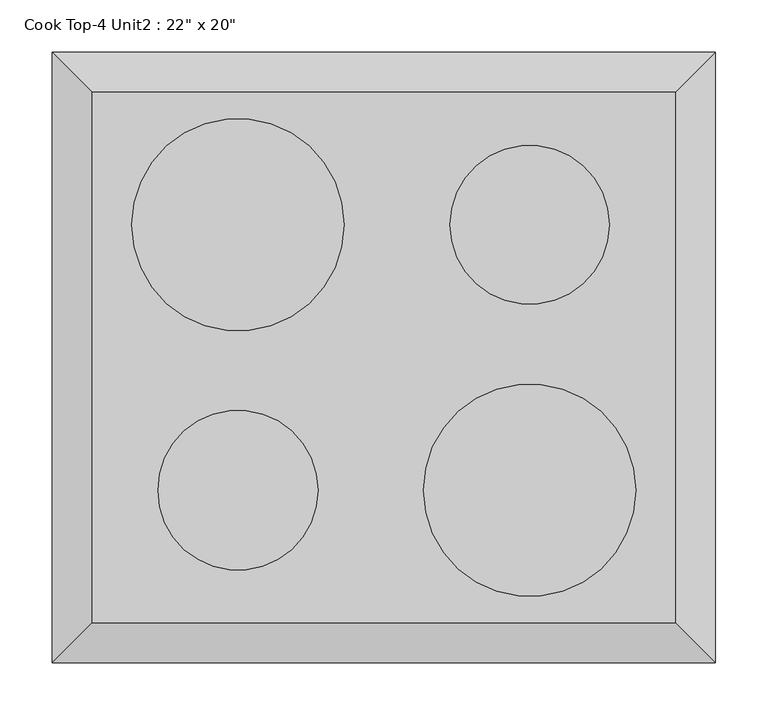
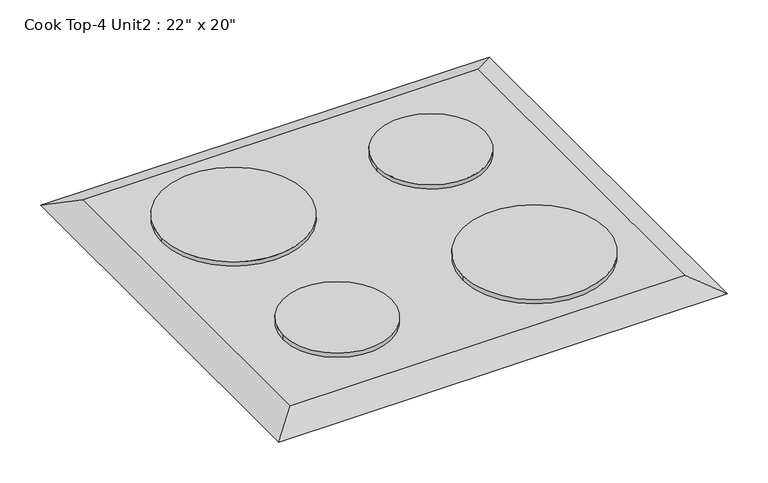
"""IFC4 building model written with IfcOpenShell, lengths in millimetres: proxy geometry."""

from ifc_helpers import new_model, si_unit, point, frame, frame_2d, origin, place, context, project, spatial, circle_curve, trimmed, segment, composite_curve, outline, extrude, faceted_brep, source, transform, mapped, element, save


def proxy_dfcd9396(model_context):
    return source(origin(), model_context, "Body", "SolidModel", [
        extrude(outline(composite_curve([segment(trimmed(circle_curve(frame_2d((-139.7, -127.0)), 76.5869489), [point((-63.1130511, -127.0))], [point((-216.2869489, -127.0))], False, "CARTESIAN"), True, "CONTINUOUS"), segment(trimmed(circle_curve(frame_2d((-139.7, -127.0)), 76.5869489), [point((-216.2869489, -127.0))], [point((-63.1130511, -127.0))], False, "CARTESIAN"), True, "CONTINUOUS")], self_intersect=False)), frame((0.0, 0.0, 918.0), z_axis=(0.0, 0.0, 1.0), x_axis=(1.0, 0.0, 0.0)), (0.0, 0.0, 1.0), 6.35),
        extrude(outline(composite_curve([segment(trimmed(circle_curve(frame_2d((139.7, 127.0)), 76.2), [point((215.9, 127.0))], [point((63.5, 127.0))], False, "CARTESIAN"), True, "CONTINUOUS"), segment(trimmed(circle_curve(frame_2d((139.7, 127.0)), 76.2), [point((63.5, 127.0))], [point((215.9, 127.0))], False, "CARTESIAN"), True, "CONTINUOUS")], self_intersect=False)), frame((0.0, 0.0, 918.0), z_axis=(0.0, 0.0, 1.0), x_axis=(1.0, 0.0, 0.0)), (0.0, 0.0, 1.0), 6.35),
        extrude(outline(composite_curve([segment(trimmed(circle_curve(frame_2d((139.7, -127.0)), 101.6), [point((38.1, -127.0))], [point((241.3, -127.0))], False, "CARTESIAN"), True, "CONTINUOUS"), segment(trimmed(circle_curve(frame_2d((139.7, -127.0)), 101.6), [point((241.3, -127.0))], [point((38.1, -127.0))], False, "CARTESIAN"), True, "CONTINUOUS")], self_intersect=False)), frame((0.0, 0.0, 918.0), z_axis=(0.0, 0.0, 1.0), x_axis=(1.0, 0.0, 0.0)), (0.0, 0.0, 1.0), 6.35),
        faceted_brep([(279.4, -254.0, 918.0), (279.4, 254.0, 918.0), (-279.4, 254.0, 918.0), (-279.4, -254.0, 918.0), (317.5, -292.1, 900.0), (-317.5, -292.1, 900.0), (-317.5, 292.1, 900.0), (317.5, 292.1, 900.0)], [[[0, 1, 2, 3]], [[4, 5, 6, 7]], [[4, 0, 3, 5]], [[5, 3, 2, 6]], [[6, 2, 1, 7]], [[7, 1, 0, 4]]]),
        extrude(outline(composite_curve([segment(trimmed(circle_curve(frame_2d((-139.7, 127.0)), 101.6), [point((-38.1, 127.0))], [point((-241.3, 127.0))], False, "CARTESIAN"), True, "CONTINUOUS"), segment(trimmed(circle_curve(frame_2d((-139.7, 127.0)), 101.6), [point((-241.3, 127.0))], [point((-38.1, 127.0))], False, "CARTESIAN"), True, "CONTINUOUS")], self_intersect=False)), frame((0.0, 0.0, 918.0), z_axis=(0.0, 0.0, 1.0), x_axis=(1.0, 0.0, 0.0)), (0.0, 0.0, 1.0), 6.35),
    ])


if __name__ == "__main__":
    model = new_model("IFC4")
    model_context = context("Model", 3, world=origin())
    ifc_project = project(units=[si_unit("LENGTHUNIT", "METRE", prefix="MILLI")], contexts=[model_context])
    site = spatial("IfcSite", under=ifc_project)
    building = spatial("IfcBuilding", under=site)
    placement = place(None, origin())
    proxy_shape = proxy_dfcd9396(model_context)
    element("IfcBuildingElementProxy", 1, Name="Cook Top-4 Unit2 : 22\" x 20\"", ObjectType="Cook Top-4 Unit2 : 22\" x 20\"", at=placement, inside=building, context=model_context, shape_type="MappedRepresentation", body=[
        mapped(proxy_shape, transform((0.0, 0.0, 0.0), x_axis=(1.0, 0.0, 0.0), y_axis=(0.0, 1.0, 0.0), z_axis=(0.0, 0.0, 1.0))),
    ])
    save(model, "model.ifc")

# Revit data of these elements
# Type "Cook Top-4 Unit2 : 22\" x 20\""
#   Depth = 1' - 8"
#   Width = 1' - 10"
#   Burner Material = Steel, Chrome Plated
#   Cooktop Material = Steel, Polished
#   Default Elevation = 0
#   Assembly Code = ""
# Element 1 (IfcBuildingElementProxy, "Cook Top-4 Unit2 : 22\" x 20\"")
#   Materials on its faces: "Steel, Chrome Plated", "Steel, Polished"
# Materials
#   "Steel, Chrome Plated": class "Metal", colour RGB 17 17 17, transparency 0, Description = "Chromiuim plated steel", Cost = 0
#   "Steel, Polished": class "Metal", colour RGB 57 57 57, transparency 0, Description = "Polished steel", Cost = 0
